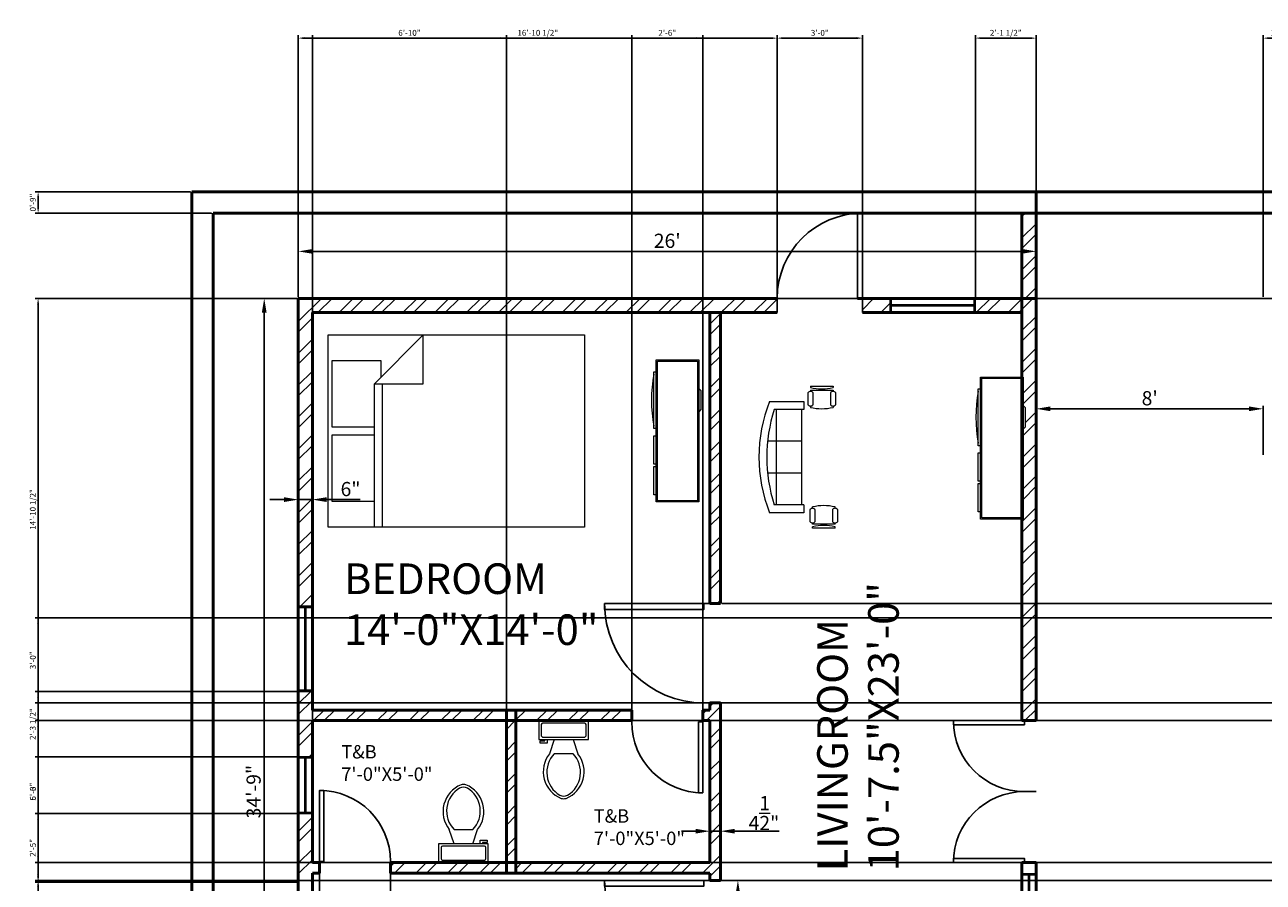
# Model space of a CAD drawing. Units: inches. Extents: x -12550 to 6516, y 1273 to 18700.
# Tile 5 of 19: x 1902 to 2426, y 2226 to 2589. Entities that reach past the tile are written whole.
import ezdxf

# ---------------------------------------------------------------- set-up
doc = ezdxf.new("R2010")
doc.units = ezdxf.units.IN
for name, color, linetype, lineweight in [('A-ANNO-DIMS', 2, 'Continuous', 18), ('A-AREA-IDEN', 1, 'Continuous', 18), ('A-DOOR', 5, 'Continuous', 25), ('A-FURN', 8, 'Continuous', 18), ('A-GLAZ', 3, 'Continuous', 25), ('A-WALL', 7, 'Continuous', 50), ('A-WALL-PATT', 8, 'Continuous', 13)]:
    doc.layers.add(name, color=color, linetype=linetype, lineweight=lineweight)
doc.styles.get("Standard").update_dxf_attribs({"font": 'arial.ttf'})
doc.dimstyles.new('ISO-25', dxfattribs={"dimtxt": 2.5, "dimasz": 2.5, "dimexe": 1.25, "dimexo": 0.625, "dimtad": 1, "dimlunit": 4, "dimtxsty": 'Standard', "dimcen": 2.5, "dimadec": 0, "dimazin": 0, "dimtfac": 1, "dimtmove": 0, "dimatfit": 3, "dimfxl": 1, "dimarcsym": 0})
pattern_1 = [(45, (-2e-13, 567), (-6.735192, 6.735192), []), (45, (4.49, 567), (-6.735192, 6.735192), [])]

# ---------------------------------------------------------------- blocks, each defined once
blk = doc.blocks.new('*U2')
for p, q in [((0, 0), (0, -5)), ((30, 0), (30, -5))]:
    blk.add_line(p, q)
blk.add_lwpolyline([(0, 0), (0, 30), (1.75, 30), (1.75, 0)], close=True)
blk.add_arc((0, 0), 30, 0, 90)
blk = doc.blocks.new('Bed - Queen')
for p, q in [((0, -80.00003), (0, 0)), ((0, 0), (59.99999, 0)), ((59.99999, 0), (59.99999, -80.00003)), ((7.99999, -1.2), (28.79998, -1.2)), ((7.99999, -14.4), (7.99999, -1.2)), ((28.79998, -1.2), (28.79998, -14.4)), ((31.19999, -1.2), (51.99999, -1.2)), ((31.19999, -14.4), (31.19999, -1.2)), ((51.99999, -1.2), (51.99999, -16.4)), ((0, -14.4), (44.8, -14.4)), ((59.99999, -29.6), (44.8, -14.4)), ((44.8, -14.4), (44.8, -29.6)), ((44.8, -16.8), (0, -16.8)), ((51.99999, -16.4), (46.79936, -16.4)), ((44.8, -29.6), (59.99999, -29.6)), ((59.99999, -80.00003), (0, -80.00003))]:
    blk.add_line(p, q)
blk = doc.blocks.new('Toilet - top')
for p, q in [((9.5, -6), (9.5, -2)), ((-10, -8.5), (-8, -8.5)), ((-10, -9.5), (-10, -8.5)), ((-7, -9.5), (-10, -9.5)), ((-8, -8.5), (-8, -8)), ((-7, -8), (-7, -9.5)), ((-4, -8), (-6, -14)), ((4, -8), (6, -14)), ((4, -14), (-4, -14))]:
    blk.add_line(p, q)
blk.add_lwpolyline([(10.5, -8), (10.5, 0), (-10.5, 0), (-10.5, -8)], close=True)
for points in [[(-9.5, -2), (-9.5, -6)], [(8.5, -1), (-8.5, -1)], [(-8.5, -7), (8.5, -7)]]:
    blk.add_lwpolyline(points)
for centre, radius, start, end in [((-8.62, -1.88), 0.884, 81.8699, 188.1301), ((8.62, -1.88), 0.884, 351.8699, 98.1301), ((-8.62, -6.12), 0.884, 171.8699, 278.1301), ((8.62, -6.12), 0.884, 261.8699, 8.1301), ((3.52, -21.58), 12.17, 141.4691, 247.9714), ((4.2, -21.82), 11.33, 136.3677, 238.9468), ((-3.52, -21.58), 12.17, 292.0284, 38.5307), ((-4.2, -21.82), 11.33, 301.053, 43.6321), ((0, -27.88), 4, 245.7318, 294.2682), ((0, -29), 4, 254.8605, 285.1395)]:
    blk.add_arc(centre, radius, start, end)
blk = doc.blocks.new('Entertainment Center')
for p, q in [((-4, 0), (-5, -1)), ((4, 0), (-4, 0)), ((5, -1), (4, 0)), ((-17, -19), (-17, -1)), ((-17, -1), (43, -1)), ((-16.5, -18.5), (-16.5, -1.5)), ((-16.5, -1.5), (42.5, -1.5)), ((42.5, -1.5), (42.5, -18.5)), ((43, -1), (43, -19)), ((43, -19), (-17, -19)), ((42.5, -18.5), (-16.5, -18.5)), ((-12, -20), (-12, -19)), ((12, -20), (-12, -20)), ((12, -19), (12, -20)), ((15, -20), (15, -19)), ((27, -20), (15, -20)), ((27, -19), (27, -20)), ((28, -20), (28, -19)), ((40, -20), (28, -20)), ((40, -19), (40, -20))]:
    blk.add_line(p, q)
blk.add_arc((0, 40), 61, 259.6111, 280.3889)
blk = doc.blocks.new('Sofa - Roundback 7 ft.')
for p, q in [((-12.00002, -32.4421), (-12.00003, -6.5971)), ((11.99997, -32.4421), (11.99998, -6.5971)), ((-36.000027, -34), (-36.000027, -11.4696)), ((-35.999844, -13.3819), (35.9998, -13.3819)), ((35.99998, -34), (35.99998, -11.4696)), ((-36.000027, -32.4421), (35.99998, -32.4421))]:
    blk.add_line(p, q)
for points in [[(-36.000027, -34), (-42.000027, -34), (-42.000027, -8)], [(41.99998, -8), (41.99998, -34), (35.99998, -34)]]:
    blk.add_lwpolyline(points)
for centre, radius, start, end in [((0, -114.25), 114.25, 68.43141, 111.5686), ((-0.00001, -127.1968), 121.1968, 72.72033, 107.2797)]:
    blk.add_arc(centre, radius, start, end)
blk = doc.blocks.new('Chair - Desk')
for p, q in [((-8.5, 0), (-8.5, -1)), ((-8.5, 0), (8.5, 0)), ((8.5, 0), (8.5, -1)), ((-10.5, -5), (-10.5, -14)), ((-8.5, -3), (-8.5, -4)), ((-8.5, -3), (8.5, -3)), ((-6.5, -14), (-6.5, -5)), ((-2, -3), (-2, -1.9355)), ((2, -1.9576), (2, -3)), ((6.5, -5), (6.5, -14)), ((8.5, -3), (8.5, -4)), ((10.5, -14), (10.5, -5)), ((-8.5, -15), (-8.5, -16)), ((8.5, -15), (8.5, -16))]:
    blk.add_line(p, q)
for centre, radius, start, end in [((-8.5, -6.5), 2.5, 36.8699, 143.1301), ((0, 34.625), 36.625, 256.5803, 283.4197), ((8.5, -6.5), 2.5, 36.8699, 143.1301), ((-8.5, -12.5), 2.5, 216.8699, 323.1301), ((0, 19.625), 36.625, 256.5803, 283.4197), ((8.5, -12.5), 2.5, 216.8699, 323.1301)]:
    blk.add_arc(centre, radius, start, end)
blk = doc.blocks.new('*D8')
at = {"layer": 'A-ANNO-DIMS', "color": 0, "lineweight": -2, "transparency": 16777216}
for p, q in [((2011.69, 2388.18), (2005.69, 2388.18)), ((2017.69, 2388.03), (2017.69, 2389.43)), ((2017.69, 2388.18), (2023.69, 2388.18)), ((2023.69, 2388.03), (2023.69, 2389.43)), ((2029.69, 2388.18), (2043.87, 2388.18))]:
    blk.add_line(p, q, dxfattribs=at)
at = {"layer": 'A-ANNO-DIMS', "color": 0, "transparency": 16777216}
for points in [[(2011.69, 2389.18), (2011.69, 2387.18), (2017.69, 2388.18)], [(2029.69, 2389.18), (2029.69, 2387.18), (2023.69, 2388.18)]]:
    blk.add_solid(points, dxfattribs=at)
at = {"layer": 'Defpoints', "color": 0, "transparency": 16777216}
for p in [(2023.69, 2388.18), (2017.69, 2387.4), (2023.69, 2387.4)]:
    blk.add_point(p, dxfattribs=at)
at = {"layer": 'A-ANNO-DIMS', "color": 0, "transparency": 16777216, "insert": (2039.78, 2391.87), "char_height": 6, "attachment_point": 5}
blk.add_mtext('6"', dxfattribs=at)
blk = doc.blocks.new('*D9')
at = {"layer": 'A-ANNO-DIMS', "color": 0, "lineweight": -2, "transparency": 16777216}
for p, q in [((2191.69, 2251.78), (2191.69, 2246.78)), ((2196.19, 2251.78), (2196.19, 2246.78)), ((2185.69, 2248.03), (2179.69, 2248.03)), ((2191.69, 2248.03), (2196.19, 2248.03)), ((2202.19, 2248.03), (2220.95, 2248.03))]:
    blk.add_line(p, q, dxfattribs=at)
at = {"layer": 'A-ANNO-DIMS', "color": 0, "transparency": 16777216}
for points in [[(2185.69, 2249.03), (2185.69, 2247.03), (2191.69, 2248.03)], [(2202.19, 2249.03), (2202.19, 2247.03), (2196.19, 2248.03)]]:
    blk.add_solid(points, dxfattribs=at)
at = {"layer": 'Defpoints', "color": 0, "transparency": 16777216}
for p in [(2191.69, 2252.41), (2196.19, 2252.41), (2196.19, 2248.03)]:
    blk.add_point(p, dxfattribs=at)
at = {"layer": 'A-ANNO-DIMS', "color": 0, "transparency": 16777216, "insert": (2214.57, 2255.68), "char_height": 6, "attachment_point": 5}
blk.add_mtext('4{\\H1x;\\S1/2;}"', dxfattribs=at)
blk = doc.blocks.new('*D10')
at = {"layer": 'A-ANNO-DIMS', "color": 0, "lineweight": -2, "transparency": 16777216}
for p, q in [((2196.81, 2227.25), (2204.82, 2227.25)), ((2203.57, 2221.25), (2203.57, 2191.25)), ((2196.81, 2185.25), (2204.82, 2185.25))]:
    blk.add_line(p, q, dxfattribs=at)
at = {"layer": 'A-ANNO-DIMS', "color": 0, "transparency": 16777216}
for points in [[(2202.57, 2221.25), (2204.57, 2221.25), (2203.57, 2227.25)], [(2202.57, 2191.25), (2204.57, 2191.25), (2203.57, 2185.25)]]:
    blk.add_solid(points, dxfattribs=at)
at = {"layer": 'Defpoints', "color": 0, "transparency": 16777216}
for p in [(2196.19, 2227.25), (2196.19, 2185.25), (2203.57, 2185.25)]:
    blk.add_point(p, dxfattribs=at)
at = {"layer": 'A-ANNO-DIMS', "color": 0, "transparency": 16777216, "insert": (2199.88, 2206.25), "char_height": 6, "attachment_point": 5, "rotation": 90}
blk.add_mtext('3\'-6"', dxfattribs=at)
blk = doc.blocks.new('*D15')
at = {"layer": 'A-ANNO-DIMS', "color": 0, "lineweight": -2, "transparency": 16777216}
for p, q in [((2017.06, 2473.25), (2002.03, 2473.25)), ((2003.28, 2467.25), (2003.28, 2062.25)), ((2017.06, 2056.25), (2002.03, 2056.25))]:
    blk.add_line(p, q, dxfattribs=at)
at = {"layer": 'A-ANNO-DIMS', "color": 0, "transparency": 16777216}
for points in [[(2002.28, 2467.25), (2004.28, 2467.25), (2003.28, 2473.25)], [(2002.28, 2062.25), (2004.28, 2062.25), (2003.28, 2056.25)]]:
    blk.add_solid(points, dxfattribs=at)
at = {"layer": 'Defpoints', "color": 0, "transparency": 16777216}
for p in [(2017.69, 2473.25), (2003.28, 2056.25), (2017.69, 2056.25)]:
    blk.add_point(p, dxfattribs=at)
at = {"layer": 'A-ANNO-DIMS', "color": 0, "transparency": 16777216, "insert": (1999.59, 2264.75), "char_height": 6, "attachment_point": 5, "rotation": 90}
blk.add_mtext('34\'-9"', dxfattribs=at)
blk = doc.blocks.new('*D18')
at = {"layer": 'A-ANNO-DIMS', "color": 0, "lineweight": -2, "transparency": 16777216}
for p, q in [((2017.69, 2473.87), (2017.69, 2494.36)), ((2023.69, 2493.11), (2323.69, 2493.11)), ((2329.69, 2473.87), (2329.69, 2494.36))]:
    blk.add_line(p, q, dxfattribs=at)
at = {"layer": 'A-ANNO-DIMS', "color": 0, "transparency": 16777216}
for points in [[(2023.69, 2494.11), (2023.69, 2492.11), (2017.69, 2493.11)], [(2323.69, 2494.11), (2323.69, 2492.11), (2329.69, 2493.11)]]:
    blk.add_solid(points, dxfattribs=at)
at = {"layer": 'Defpoints', "color": 0, "transparency": 16777216}
for p in [(2329.69, 2493.11), (2017.69, 2473.25), (2329.69, 2473.25)]:
    blk.add_point(p, dxfattribs=at)
at = {"layer": 'A-ANNO-DIMS', "color": 0, "transparency": 16777216, "insert": (2173.69, 2496.8), "char_height": 6, "attachment_point": 5}
blk.add_mtext("26'", dxfattribs=at)
blk = doc.blocks.new('*D19')
at = {"layer": 'A-ANNO-DIMS', "color": 0, "lineweight": -2, "transparency": 16777216}
for p, q in [((2329.69, 2407.12), (2329.69, 2427.81)), ((2335.69, 2426.56), (2419.69, 2426.56)), ((2425.69, 2407.12), (2425.69, 2427.81))]:
    blk.add_line(p, q, dxfattribs=at)
at = {"layer": 'A-ANNO-DIMS', "color": 0, "transparency": 16777216}
for points in [[(2335.69, 2427.56), (2335.69, 2425.56), (2329.69, 2426.56)], [(2419.69, 2427.56), (2419.69, 2425.56), (2425.69, 2426.56)]]:
    blk.add_solid(points, dxfattribs=at)
at = {"layer": 'Defpoints', "color": 0, "transparency": 16777216}
for p in [(2425.69, 2426.56), (2329.69, 2406.5), (2425.69, 2406.5)]:
    blk.add_point(p, dxfattribs=at)
at = {"layer": 'A-ANNO-DIMS', "color": 0, "transparency": 16777216, "insert": (2377.69, 2430.25), "char_height": 6, "attachment_point": 5}
blk.add_mtext("8'", dxfattribs=at)
blk = doc.blocks.new('WIN-3FT')
for p, q in [((0, 0), (0, 6)), ((0, 6), (36.02, 6)), ((0.5, 0), (0.5, 6)), ((35.52, 6), (35.52, 0)), ((36.02, 6), (36.02, 0)), ((36.02, 0), (0, 0)), ((35.52, 3.2), (0.5, 3.2)), ((35.52, 2.8), (0.5, 2.8))]:
    blk.add_line(p, q)
blk = doc.blocks.new('WIN-2FT')
for p, q in [((0, 0), (0, 24.02)), ((0, 24.02), (6, 24.02)), ((0, 23.52), (6, 23.52)), ((2.8, 0.5), (2.8, 23.52)), ((3.2, 0.5), (3.2, 23.52)), ((6, 24.02), (6, 0)), ((6, 0.5), (0, 0.5)), ((6, 0), (0, 0))]:
    blk.add_line(p, q)
blk = doc.blocks.new('*D102')
at = {"layer": 'A-ANNO-DIMS', "color": 0, "lineweight": -2, "transparency": 16777216}
for p, q in [((1972.06, 2518.25), (1906.44, 2518.25)), ((1907.69, 2515.75), (1907.69, 2511.75)), ((1981.06, 2509.25), (1906.44, 2509.25))]:
    blk.add_line(p, q, dxfattribs=at)
at = {"layer": 'A-ANNO-DIMS', "color": 0, "transparency": 16777216}
for points in [[(1907.27, 2515.75), (1908.11, 2515.75), (1907.69, 2518.25)], [(1907.27, 2511.75), (1908.11, 2511.75), (1907.69, 2509.25)]]:
    blk.add_solid(points, dxfattribs=at)
at = {"layer": 'Defpoints', "color": 0, "transparency": 16777216}
for p in [(1972.69, 2518.25), (1907.69, 2509.25), (1981.69, 2509.25)]:
    blk.add_point(p, dxfattribs=at)
at = {"layer": 'A-ANNO-DIMS', "color": 0, "transparency": 16777216, "insert": (1905.79, 2513.75), "char_height": 2.5, "attachment_point": 5, "rotation": 90}
blk.add_mtext('0\'-9"', dxfattribs=at)
blk = doc.blocks.new('*D130')
at = {"layer": 'A-ANNO-DIMS', "color": 0, "lineweight": -2, "transparency": 16777216}
for p, q in [((2017.69, 2473.87), (2017.69, 2584.5)), ((2020.19, 2583.25), (2217.69, 2583.25)), ((2220.19, 2473.87), (2220.19, 2584.5))]:
    blk.add_line(p, q, dxfattribs=at)
at = {"layer": 'A-ANNO-DIMS', "color": 0, "transparency": 16777216}
for points in [[(2020.19, 2583.66), (2020.19, 2582.83), (2017.69, 2583.25)], [(2217.69, 2583.66), (2217.69, 2582.83), (2220.19, 2583.25)]]:
    blk.add_solid(points, dxfattribs=at)
at = {"layer": 'Defpoints', "color": 0, "transparency": 16777216}
for p in [(2220.19, 2583.25), (2017.69, 2473.25), (2220.19, 2473.25)]:
    blk.add_point(p, dxfattribs=at)
at = {"layer": 'A-ANNO-DIMS', "color": 0, "transparency": 16777216, "insert": (2118.94, 2585.16), "char_height": 2.5, "attachment_point": 5}
blk.add_mtext('16\'-10 1/2"', dxfattribs=at)
blk = doc.blocks.new('*D131')
at = {"layer": 'A-ANNO-DIMS', "color": 0, "lineweight": -2, "transparency": 16777216}
for p, q in [((2220.19, 2473.87), (2220.19, 2584.5)), ((2222.69, 2583.25), (2253.69, 2583.25)), ((2256.19, 2473.87), (2256.19, 2584.5))]:
    blk.add_line(p, q, dxfattribs=at)
at = {"layer": 'A-ANNO-DIMS', "color": 0, "transparency": 16777216}
for points in [[(2222.69, 2583.66), (2222.69, 2582.83), (2220.19, 2583.25)], [(2253.69, 2583.66), (2253.69, 2582.83), (2256.19, 2583.25)]]:
    blk.add_solid(points, dxfattribs=at)
at = {"layer": 'Defpoints', "color": 0, "transparency": 16777216}
for p in [(2256.19, 2583.25), (2220.19, 2473.25), (2256.19, 2473.25)]:
    blk.add_point(p, dxfattribs=at)
at = {"layer": 'A-ANNO-DIMS', "color": 0, "transparency": 16777216, "insert": (2238.19, 2585.15), "char_height": 2.5, "attachment_point": 5}
blk.add_mtext('3\'-0"', dxfattribs=at)
blk = doc.blocks.new('*D132')
at = {"layer": 'A-ANNO-DIMS', "color": 0, "lineweight": -2, "transparency": 16777216}
for p, q in [((2303.96, 2473.87), (2303.96, 2584.5)), ((2306.46, 2583.25), (2327.19, 2583.25)), ((2329.69, 2473.87), (2329.69, 2584.5))]:
    blk.add_line(p, q, dxfattribs=at)
at = {"layer": 'A-ANNO-DIMS', "color": 0, "transparency": 16777216}
for points in [[(2306.46, 2583.66), (2306.46, 2582.83), (2303.96, 2583.25)], [(2327.19, 2583.66), (2327.19, 2582.83), (2329.69, 2583.25)]]:
    blk.add_solid(points, dxfattribs=at)
at = {"layer": 'Defpoints', "color": 0, "transparency": 16777216}
for p in [(2329.69, 2583.25), (2303.96, 2473.25), (2329.69, 2473.25)]:
    blk.add_point(p, dxfattribs=at)
at = {"layer": 'A-ANNO-DIMS', "color": 0, "transparency": 16777216, "insert": (2316.82, 2585.16), "char_height": 2.5, "attachment_point": 5}
blk.add_mtext('2\'-1 1/2"', dxfattribs=at)
blk = doc.blocks.new('*D134')
at = {"layer": 'A-ANNO-DIMS', "color": 0, "lineweight": -2, "transparency": 16777216}
for p, q in [((2017.06, 2255.45), (1906.44, 2255.45)), ((1907.69, 2228.95), (1907.69, 2252.95)), ((2017.06, 2226.45), (1906.44, 2226.45))]:
    blk.add_line(p, q, dxfattribs=at)
at = {"layer": 'A-ANNO-DIMS', "color": 0, "transparency": 16777216}
for points in [[(1907.27, 2252.95), (1908.11, 2252.95), (1907.69, 2255.45)], [(1907.27, 2228.95), (1908.11, 2228.95), (1907.69, 2226.45)]]:
    blk.add_solid(points, dxfattribs=at)
at = {"layer": 'Defpoints', "color": 0, "transparency": 16777216}
for p in [(1907.69, 2255.45), (2017.69, 2255.45), (2017.69, 2226.45)]:
    blk.add_point(p, dxfattribs=at)
at = {"layer": 'A-ANNO-DIMS', "color": 0, "transparency": 16777216, "insert": (1905.79, 2240.95), "char_height": 2.5, "attachment_point": 5, "rotation": 90}
blk.add_mtext('2\'-5"', dxfattribs=at)
blk = doc.blocks.new('*D135')
at = {"layer": 'A-ANNO-DIMS', "color": 0, "lineweight": -2, "transparency": 16777216}
for p, q in [((2017.06, 2307.12), (1906.44, 2307.12)), ((1907.69, 2281.97), (1907.69, 2304.62)), ((2017.06, 2279.47), (1906.44, 2279.47))]:
    blk.add_line(p, q, dxfattribs=at)
at = {"layer": 'A-ANNO-DIMS', "color": 0, "transparency": 16777216}
for points in [[(1907.27, 2304.62), (1908.11, 2304.62), (1907.69, 2307.12)], [(1907.27, 2281.97), (1908.11, 2281.97), (1907.69, 2279.47)]]:
    blk.add_solid(points, dxfattribs=at)
at = {"layer": 'Defpoints', "color": 0, "transparency": 16777216}
for p in [(1907.69, 2307.12), (2017.69, 2307.12), (2017.69, 2279.47)]:
    blk.add_point(p, dxfattribs=at)
at = {"layer": 'A-ANNO-DIMS', "color": 0, "transparency": 16777216, "insert": (1905.77, 2293.29), "char_height": 2.5, "attachment_point": 5, "rotation": 90}
blk.add_mtext('2\'-3 1/2"', dxfattribs=at)
blk = doc.blocks.new('*D139')
at = {"layer": 'A-ANNO-DIMS', "color": 0, "lineweight": -2, "transparency": 16777216}
for p, q in [((2196.81, 2302.25), (2848.94, 2302.25)), ((2847.69, 2229.75), (2847.69, 2299.75)), ((2196.81, 2227.25), (2848.94, 2227.25))]:
    blk.add_line(p, q, dxfattribs=at)
at = {"layer": 'A-ANNO-DIMS', "color": 0, "transparency": 16777216}
for points in [[(2847.27, 2299.75), (2848.11, 2299.75), (2847.69, 2302.25)], [(2847.27, 2229.75), (2848.11, 2229.75), (2847.69, 2227.25)]]:
    blk.add_solid(points, dxfattribs=at)
at = {"layer": 'Defpoints', "color": 0, "transparency": 16777216}
for p in [(2196.19, 2302.25), (2847.69, 2302.25), (2196.19, 2227.25)]:
    blk.add_point(p, dxfattribs=at)
at = {"layer": 'A-ANNO-DIMS', "color": 0, "transparency": 16777216, "insert": (2845.79, 2264.75), "char_height": 2.5, "attachment_point": 5, "rotation": 90}
blk.add_mtext('6\'-3"', dxfattribs=at)
blk = doc.blocks.new('*D140')
at = {"layer": 'A-ANNO-DIMS', "color": 0, "lineweight": -2, "transparency": 16777216}
for p, q in [((2196.81, 2344.25), (2848.94, 2344.25)), ((2847.69, 2304.75), (2847.69, 2341.75)), ((2196.81, 2302.25), (2848.94, 2302.25))]:
    blk.add_line(p, q, dxfattribs=at)
at = {"layer": 'A-ANNO-DIMS', "color": 0, "transparency": 16777216}
for points in [[(2847.27, 2341.75), (2848.11, 2341.75), (2847.69, 2344.25)], [(2847.27, 2304.75), (2848.11, 2304.75), (2847.69, 2302.25)]]:
    blk.add_solid(points, dxfattribs=at)
at = {"layer": 'Defpoints', "color": 0, "transparency": 16777216}
for p in [(2196.19, 2344.25), (2847.69, 2344.25), (2196.19, 2302.25)]:
    blk.add_point(p, dxfattribs=at)
at = {"layer": 'A-ANNO-DIMS', "color": 0, "transparency": 16777216, "insert": (2845.79, 2323.25), "char_height": 2.5, "attachment_point": 5, "rotation": 90}
blk.add_mtext('3\'-6"', dxfattribs=at)
blk = doc.blocks.new('*D141')
at = {"layer": 'A-ANNO-DIMS', "color": 0, "lineweight": -2, "transparency": 16777216}
for p, q in [((2158.69, 2295.37), (2158.69, 2584.5)), ((2161.19, 2583.25), (2186.19, 2583.25)), ((2188.69, 2295.37), (2188.69, 2584.5))]:
    blk.add_line(p, q, dxfattribs=at)
at = {"layer": 'A-ANNO-DIMS', "color": 0, "transparency": 16777216}
for points in [[(2161.19, 2583.66), (2161.19, 2582.83), (2158.69, 2583.25)], [(2186.19, 2583.66), (2186.19, 2582.83), (2188.69, 2583.25)]]:
    blk.add_solid(points, dxfattribs=at)
at = {"layer": 'Defpoints', "color": 0, "transparency": 16777216}
for p in [(2188.69, 2583.25), (2158.69, 2294.75), (2188.69, 2294.75)]:
    blk.add_point(p, dxfattribs=at)
at = {"layer": 'A-ANNO-DIMS', "color": 0, "transparency": 16777216, "insert": (2173.69, 2585.15), "char_height": 2.5, "attachment_point": 5}
blk.add_mtext('2\'-6"', dxfattribs=at)
blk = doc.blocks.new('*D142')
at = {"layer": 'A-ANNO-DIMS', "color": 0, "lineweight": -2, "transparency": 16777216}
for p, q in [((2026.69, 2234.12), (2026.69, 1378)), ((2056.69, 2234.12), (2056.69, 1378)), ((2029.19, 1379.25), (2054.19, 1379.25))]:
    blk.add_line(p, q, dxfattribs=at)
at = {"layer": 'A-ANNO-DIMS', "color": 0, "transparency": 16777216}
for points in [[(2029.19, 1379.66), (2029.19, 1378.83), (2026.69, 1379.25)], [(2054.19, 1379.66), (2054.19, 1378.83), (2056.69, 1379.25)]]:
    blk.add_solid(points, dxfattribs=at)
at = {"layer": 'Defpoints', "color": 0, "transparency": 16777216}
for p in [(2026.69, 2234.75), (2056.69, 2234.75), (2056.69, 1379.25)]:
    blk.add_point(p, dxfattribs=at)
at = {"layer": 'A-ANNO-DIMS', "color": 0, "transparency": 16777216, "insert": (2041.69, 1381.15), "char_height": 2.5, "attachment_point": 5}
blk.add_mtext('2\'-6"', dxfattribs=at)
blk = doc.blocks.new('*D143')
at = {"layer": 'A-ANNO-DIMS', "color": 0, "lineweight": -2, "transparency": 16777216}
for p, q in [((2023.69, 2295.37), (2023.69, 2584.5)), ((2026.19, 2583.25), (2103.19, 2583.25)), ((2105.69, 2299.87), (2105.69, 2584.5))]:
    blk.add_line(p, q, dxfattribs=at)
at = {"layer": 'A-ANNO-DIMS', "color": 0, "transparency": 16777216}
for points in [[(2026.19, 2583.66), (2026.19, 2582.83), (2023.69, 2583.25)], [(2103.19, 2583.66), (2103.19, 2582.83), (2105.69, 2583.25)]]:
    blk.add_solid(points, dxfattribs=at)
at = {"layer": 'Defpoints', "color": 0, "transparency": 16777216}
for p in [(2105.69, 2583.25), (2105.69, 2299.25), (2023.69, 2294.75)]:
    blk.add_point(p, dxfattribs=at)
at = {"layer": 'A-ANNO-DIMS', "color": 0, "transparency": 16777216, "insert": (2064.69, 2585.15), "char_height": 2.5, "attachment_point": 5}
blk.add_mtext('6\'-10"', dxfattribs=at)
blk = doc.blocks.new('*D144')
at = {"layer": 'A-ANNO-DIMS', "color": 0, "lineweight": -2, "transparency": 16777216}
for p, q in [((2330.31, 2294.75), (2848.94, 2294.75)), ((2847.69, 2237.25), (2847.69, 2292.25)), ((2330.31, 2234.75), (2848.94, 2234.75))]:
    blk.add_line(p, q, dxfattribs=at)
at = {"layer": 'A-ANNO-DIMS', "color": 0, "transparency": 16777216}
for points in [[(2847.27, 2292.25), (2848.11, 2292.25), (2847.69, 2294.75)], [(2847.27, 2237.25), (2848.11, 2237.25), (2847.69, 2234.75)]]:
    blk.add_solid(points, dxfattribs=at)
at = {"layer": 'Defpoints', "color": 0, "transparency": 16777216}
for p in [(2329.69, 2294.75), (2847.69, 2294.75), (2329.69, 2234.75)]:
    blk.add_point(p, dxfattribs=at)
at = {"layer": 'A-ANNO-DIMS', "color": 0, "transparency": 16777216, "insert": (2845.79, 2264.75), "char_height": 2.5, "attachment_point": 5, "rotation": 90}
blk.add_mtext('5\'-0"', dxfattribs=at)
blk = doc.blocks.new('*D146')
at = {"layer": 'A-ANNO-DIMS', "color": 0, "lineweight": -2, "transparency": 16777216}
for p, q in [((2330.31, 2473.25), (2848.94, 2473.25)), ((2847.69, 2297.25), (2847.69, 2470.75)), ((2330.31, 2294.75), (2848.94, 2294.75))]:
    blk.add_line(p, q, dxfattribs=at)
at = {"layer": 'A-ANNO-DIMS', "color": 0, "transparency": 16777216}
for points in [[(2847.27, 2470.75), (2848.11, 2470.75), (2847.69, 2473.25)], [(2847.27, 2297.25), (2848.11, 2297.25), (2847.69, 2294.75)]]:
    blk.add_solid(points, dxfattribs=at)
at = {"layer": 'Defpoints', "color": 0, "transparency": 16777216}
for p in [(2329.69, 2473.25), (2847.69, 2473.25), (2329.69, 2294.75)]:
    blk.add_point(p, dxfattribs=at)
at = {"layer": 'A-ANNO-DIMS', "color": 0, "transparency": 16777216, "insert": (2845.77, 2384), "char_height": 2.5, "attachment_point": 5, "rotation": 90}
blk.add_mtext('14\'-10 1/2"', dxfattribs=at)
blk = doc.blocks.new('*D149')
at = {"layer": 'A-ANNO-DIMS', "color": 0, "lineweight": -2, "transparency": 16777216}
for p, q in [((2425.69, 2473.87), (2425.69, 2584.5)), ((2428.19, 2583.25), (2436.95, 2583.25)), ((2439.45, 2473.87), (2439.45, 2584.5))]:
    blk.add_line(p, q, dxfattribs=at)
at = {"layer": 'A-ANNO-DIMS', "color": 0, "transparency": 16777216}
for points in [[(2428.19, 2583.66), (2428.19, 2582.83), (2425.69, 2583.25)], [(2436.95, 2583.66), (2436.95, 2582.83), (2439.45, 2583.25)]]:
    blk.add_solid(points, dxfattribs=at)
at = {"layer": 'Defpoints', "color": 0, "transparency": 16777216}
for p in [(2439.45, 2583.25), (2425.69, 2473.25), (2439.45, 2473.25)]:
    blk.add_point(p, dxfattribs=at)
at = {"layer": 'A-ANNO-DIMS', "color": 0, "transparency": 16777216, "insert": (2432.57, 2585.13), "char_height": 2.5, "attachment_point": 5}
blk.add_mtext('1\'-2"', dxfattribs=at)
blk = doc.blocks.new('*D158')
at = {"layer": 'A-ANNO-DIMS', "color": 0, "lineweight": -2, "transparency": 16777216}
for p, q in [((2558.56, 2227.25), (1906.44, 2227.25)), ((1907.69, 2193.75), (1907.69, 2224.75)), ((2558.56, 2191.25), (1906.44, 2191.25))]:
    blk.add_line(p, q, dxfattribs=at)
at = {"layer": 'A-ANNO-DIMS', "color": 0, "transparency": 16777216}
for points in [[(1907.27, 2224.75), (1908.11, 2224.75), (1907.69, 2227.25)], [(1907.27, 2193.75), (1908.11, 2193.75), (1907.69, 2191.25)]]:
    blk.add_solid(points, dxfattribs=at)
at = {"layer": 'Defpoints', "color": 0, "transparency": 16777216}
for p in [(1907.69, 2227.25), (2559.19, 2227.25), (2559.19, 2191.25)]:
    blk.add_point(p, dxfattribs=at)
at = {"layer": 'A-ANNO-DIMS', "color": 0, "transparency": 16777216, "insert": (1905.79, 2209.25), "char_height": 2.5, "attachment_point": 5, "rotation": 90}
blk.add_mtext('3\'-0"', dxfattribs=at)
blk = doc.blocks.new('*D159')
at = {"layer": 'A-ANNO-DIMS', "color": 0, "lineweight": -2, "transparency": 16777216}
for p, q in [((2558.56, 2302.25), (1906.44, 2302.25)), ((1907.69, 2229.75), (1907.69, 2299.75)), ((2558.56, 2227.25), (1906.44, 2227.25))]:
    blk.add_line(p, q, dxfattribs=at)
at = {"layer": 'A-ANNO-DIMS', "color": 0, "transparency": 16777216}
for points in [[(1907.27, 2299.75), (1908.11, 2299.75), (1907.69, 2302.25)], [(1907.27, 2229.75), (1908.11, 2229.75), (1907.69, 2227.25)]]:
    blk.add_solid(points, dxfattribs=at)
at = {"layer": 'Defpoints', "color": 0, "transparency": 16777216}
for p in [(1907.69, 2302.25), (2559.19, 2302.25), (2559.19, 2227.25)]:
    blk.add_point(p, dxfattribs=at)
at = {"layer": 'A-ANNO-DIMS', "color": 0, "transparency": 16777216, "insert": (1905.79, 2264.75), "char_height": 2.5, "attachment_point": 5, "rotation": 90}
blk.add_mtext('6\'-3"', dxfattribs=at)
blk = doc.blocks.new('*D160')
at = {"layer": 'A-ANNO-DIMS', "color": 0, "lineweight": -2, "transparency": 16777216}
for p, q in [((2558.56, 2338.25), (1906.44, 2338.25)), ((1907.69, 2304.75), (1907.69, 2335.75)), ((2558.56, 2302.25), (1906.44, 2302.25))]:
    blk.add_line(p, q, dxfattribs=at)
at = {"layer": 'A-ANNO-DIMS', "color": 0, "transparency": 16777216}
for points in [[(1907.27, 2335.75), (1908.11, 2335.75), (1907.69, 2338.25)], [(1907.27, 2304.75), (1908.11, 2304.75), (1907.69, 2302.25)]]:
    blk.add_solid(points, dxfattribs=at)
at = {"layer": 'Defpoints', "color": 0, "transparency": 16777216}
for p in [(1907.69, 2338.25), (2559.19, 2338.25), (2559.19, 2302.25)]:
    blk.add_point(p, dxfattribs=at)
at = {"layer": 'A-ANNO-DIMS', "color": 0, "transparency": 16777216, "insert": (1905.79, 2320.25), "char_height": 2.5, "attachment_point": 5, "rotation": 90}
blk.add_mtext('3\'-0"', dxfattribs=at)
blk = doc.blocks.new('*D164')
at = {"layer": 'A-ANNO-DIMS', "color": 0, "lineweight": -2, "transparency": 16777216}
for p, q in [((2425.06, 2294.75), (1906.44, 2294.75)), ((1907.69, 2237.25), (1907.69, 2292.25)), ((2425.06, 2234.75), (1906.44, 2234.75))]:
    blk.add_line(p, q, dxfattribs=at)
at = {"layer": 'A-ANNO-DIMS', "color": 0, "transparency": 16777216}
for points in [[(1907.27, 2292.25), (1908.11, 2292.25), (1907.69, 2294.75)], [(1907.27, 2237.25), (1908.11, 2237.25), (1907.69, 2234.75)]]:
    blk.add_solid(points, dxfattribs=at)
at = {"layer": 'Defpoints', "color": 0, "transparency": 16777216}
for p in [(1907.69, 2294.75), (2425.69, 2294.75), (2425.69, 2234.75)]:
    blk.add_point(p, dxfattribs=at)
at = {"layer": 'A-ANNO-DIMS', "color": 0, "transparency": 16777216, "insert": (1905.79, 2264.75), "char_height": 2.5, "attachment_point": 5, "rotation": 90}
blk.add_mtext('5\'-0"', dxfattribs=at)
blk = doc.blocks.new('*D166')
at = {"layer": 'A-ANNO-DIMS', "color": 0, "lineweight": -2, "transparency": 16777216}
for p, q in [((2425.06, 2473.25), (1906.44, 2473.25)), ((1907.69, 2297.25), (1907.69, 2470.75)), ((2425.06, 2294.75), (1906.44, 2294.75))]:
    blk.add_line(p, q, dxfattribs=at)
at = {"layer": 'A-ANNO-DIMS', "color": 0, "transparency": 16777216}
for points in [[(1907.27, 2470.75), (1908.11, 2470.75), (1907.69, 2473.25)], [(1907.27, 2297.25), (1908.11, 2297.25), (1907.69, 2294.75)]]:
    blk.add_solid(points, dxfattribs=at)
at = {"layer": 'Defpoints', "color": 0, "transparency": 16777216}
for p in [(1907.69, 2473.25), (2425.69, 2473.25), (2425.69, 2294.75)]:
    blk.add_point(p, dxfattribs=at)
at = {"layer": 'A-ANNO-DIMS', "color": 0, "transparency": 16777216, "insert": (1905.77, 2384), "char_height": 2.5, "attachment_point": 5, "rotation": 90}
blk.add_mtext('14\'-10 1/2"', dxfattribs=at)

msp = doc.modelspace()

# ---------------------------------------------------------------- hatches: boundary and pattern name
at = {"layer": 'A-WALL-PATT'}
h = msp.add_hatch(dxfattribs=at)
h.set_pattern_fill('ANSI32', color=256)
h.paths.add_polyline_path([(2329.689, 2509.247), (2323.689, 2509.247), (2323.689, 2473.247), (2329.689, 2473.247)])
h = msp.add_hatch(dxfattribs=at)
h.set_pattern_fill('ANSI32', color=256)
h.set_pattern_definition(pattern_1)
h.paths.add_polyline_path([(2023.689, 2467.247), (2197.689, 2467.247), (2197.689, 2473.247), (2017.689, 2473.247), (2017.689, 2343.138), (2023.689, 2343.138)])
h = msp.add_hatch(dxfattribs=at)
h.set_pattern_fill('ANSI32', color=256)
h.set_pattern_definition(pattern_1)
h.paths.add_polyline_path([(2256.189, 2473.247), (2256.189, 2467.247), (2267.94, 2467.247), (2267.94, 2473.247)])
h.paths.add_polyline_path([(2220.189, 2467.247), (2220.189, 2473.247), (2197.689, 2473.247), (2197.689, 2467.247)])
h = msp.add_hatch(dxfattribs=at)
h.set_pattern_fill('ANSI32', color=256)
h.set_pattern_definition(pattern_1)
h.paths.add_polyline_path([(2329.689, 2473.247), (2303.958, 2473.247), (2303.958, 2467.247), (2323.689, 2467.247), (2323.689, 2439.972), (2324.189, 2439.972), (2324.189, 2427.972), (2325.189, 2426.972), (2325.189, 2418.972), (2324.189, 2417.972), (2324.189, 2379.972), (2323.689, 2294.747), (2324.689, 2294.747), (2329.689, 2294.747)])
h = msp.add_hatch(dxfattribs=at)
h.set_pattern_fill('ANSI32', color=256)
h.set_pattern_definition(pattern_1)
h.paths.add_polyline_path([(2196.189, 2467.247), (2191.689, 2467.247), (2191.689, 2344.247), (2196.189, 2344.247)], flags=17)
h = msp.add_hatch(dxfattribs=at)
h.set_pattern_fill('ANSI32', color=256)
h.set_pattern_definition(pattern_1)
h.paths.add_polyline_path([(2105.689, 2299.247), (2023.689, 2299.247), (2023.689, 2307.121), (2017.689, 2307.121), (2017.689, 2279.466), (2023.689, 2279.466), (2023.689, 2294.747), (2105.689, 2294.747)])
h = msp.add_hatch(dxfattribs=at)
h.set_pattern_fill('ANSI32', color=256)
h.set_pattern_definition(pattern_1)
h.paths.add_polyline_path([(2196.189, 2302.247), (2191.689, 2302.247), (2191.689, 2299.247), (2188.689, 2299.247), (2188.689, 2294.747), (2191.689, 2294.747), (2191.689, 2234.747), (2109.689, 2234.747), (2109.689, 2230.247), (2191.689, 2230.247), (2191.689, 2227.247), (2196.189, 2227.247)])
h = msp.add_hatch(dxfattribs=at)
h.set_pattern_fill('ANSI32', color=256)
h.set_pattern_definition(pattern_1)
h.paths.add_polyline_path([(2158.689, 2299.247), (2109.689, 2299.247), (2109.689, 2294.747), (2158.689, 2294.747)], flags=17)
h = msp.add_hatch(dxfattribs=at)
h.set_pattern_fill('ANSI32', color=256)
h.set_pattern_definition(pattern_1)
h.paths.add_polyline_path([(2109.689, 2294.747), (2105.689, 2294.747), (2105.689, 2234.747), (2109.689, 2234.747)])
h = msp.add_hatch(dxfattribs=at)
h.set_pattern_fill('ANSI32', color=256)
h.set_pattern_definition(pattern_1)
h.paths.add_polyline_path([(2023.689, 2255.449), (2017.689, 2255.449), (2017.689, 2226.453), (2023.689, 2226.453), (2023.689, 2230.247), (2026.689, 2230.247), (2026.689, 2234.747), (2023.689, 2234.747)])
h = msp.add_hatch(dxfattribs=at)
h.set_pattern_fill('ANSI32', color=256)
h.set_pattern_definition(pattern_1)
h.paths.add_polyline_path([(2105.689, 2234.747), (2056.689, 2234.747), (2056.689, 2230.247), (2105.689, 2230.247)])

# ---------------------------------------------------------------- linework, layer by layer
at = {"layer": 'A-WALL'}
for p, q in [((1972.689, 2518.247), (2782.689, 2518.247)), ((1972.689, 1444.247), (1972.689, 2518.247)), ((2329.689, 2294.747), (2329.689, 2518.247)), ((1981.689, 2509.247), (2773.689, 2509.247)), ((1981.689, 1453.247), (1981.689, 2509.247)), ((2554.089, 2509.247), (2254.089, 2509.247)), ((2323.689, 2294.747), (2323.689, 2509.247)), ((2017.689, 2068.324), (2017.689, 2473.247)), ((2220.189, 2473.247), (2017.689, 2473.247)), ((2329.689, 2473.247), (2254.089, 2473.247)), ((2023.689, 2299.247), (2023.689, 2467.247)), ((2220.189, 2467.247), (2023.689, 2467.247)), ((2191.689, 2344.247), (2191.689, 2467.247)), ((2196.189, 2344.247), (2196.189, 2467.247)), ((2323.689, 2467.247), (2256.189, 2467.247)), ((2196.189, 2344.247), (2191.689, 2344.247)), ((2158.689, 2299.247), (2023.689, 2299.247)), ((2105.689, 2230.247), (2105.689, 2299.247)), ((2109.689, 2230.247), (2109.689, 2299.247)), ((2158.689, 2294.747), (2158.689, 2299.247)), ((2191.689, 2299.247), (2188.689, 2299.247)), ((2191.689, 2299.247), (2188.689, 2299.247)), ((2188.689, 2299.247), (2188.689, 2294.747)), ((2191.689, 2299.247), (2191.689, 2302.247)), ((2191.689, 2299.247), (2191.689, 2302.247)), ((2191.689, 2302.247), (2196.189, 2302.247)), ((2196.189, 2227.247), (2196.189, 2302.247)), ((2158.689, 2294.747), (2023.689, 2294.747)), ((2023.689, 2234.747), (2023.689, 2294.747)), ((2191.689, 2294.747), (2188.689, 2294.747)), ((2191.689, 2234.747), (2191.689, 2294.747)), ((2329.689, 2294.747), (2323.689, 2294.747)), ((2026.689, 2234.747), (2023.689, 2234.747)), ((2026.689, 2230.247), (2026.689, 2234.747)), ((2191.689, 2234.747), (2056.689, 2234.747)), ((2056.689, 2234.747), (2191.689, 2234.747)), ((2056.689, 2234.747), (2056.689, 2230.247)), ((2329.689, 2234.747), (2323.689, 2234.747)), ((2323.689, 2062.247), (2323.689, 2234.747)), ((2329.689, 2056.247), (2329.689, 2234.747)), ((2026.689, 2230.247), (2023.689, 2230.247)), ((2023.689, 2062.247), (2023.689, 2230.247)), ((2023.689, 2230.247), (2026.689, 2230.247)), ((2191.689, 2230.247), (2056.689, 2230.247)), ((2191.689, 2227.247), (2191.689, 2230.247)), ((2196.189, 2227.247), (2191.689, 2227.247)), ((2196.189, 2230.247), (2196.189, 2227.247))]:
    msp.add_line(p, q, dxfattribs=at)

# ---------------------------------------------------------------- block references
at = {"layer": 'A-DOOR', "xscale": -1.199999999999999, "yscale": 1.199999999999999, "zscale": 1.199999999999999}
msp.add_blockref('*U2', (2256.189, 2473.247), dxfattribs=at)
at = {"layer": 'A-DOOR', "xscale": -1.4, "yscale": 1.4, "zscale": 1.4, "rotation": 90}
for p in [(2189.189, 2344.247), (2189.189, 2227.247)]:
    msp.add_blockref('*U2', p, dxfattribs=at)
at = {"layer": 'A-DOOR'}
for p, rotation in [((2188.689, 2294.247), 180), ((2324.689, 2234.747), 90)]:
    msp.add_blockref('*U2', p, dxfattribs=dict(at, rotation=rotation))
at = {"layer": 'A-DOOR', "xscale": -1, "rotation": 90}
msp.add_blockref('*U2', (2324.689, 2294.747), dxfattribs=at)
at = {"layer": 'A-DOOR'}
msp.add_blockref('*U2', (2026.689, 2235.247), dxfattribs=at)
at = {"layer": 'A-FURN'}
for name, p, xscale, yscale, zscale, rotation in [('Bed - Queen', (2030.339, 2376.493), 1.354827908062564, 1.354827908062564, 1.354827908062564, 90), ('Sofa - Roundback 7 ft.', (2212.448, 2406.138), 0.5595223685495907, 0.5595223685495907, 0.5595223685495907, 90), ('Chair - Desk', (2239.887, 2376.138), 0.5595223685495907, 0.5595223685495907, 0.5595223685495907, 180)]:
    msp.add_blockref(name, p, dxfattribs=dict(at, xscale=xscale, yscale=yscale, zscale=zscale, rotation=rotation))
for name, p, rotation in [('Entertainment Center', (2188.03, 2430.204), 270), ('Entertainment Center', (2325.189, 2422.972), 270), ('Toilet - top', (2087.536, 2234.747), 180)]:
    msp.add_blockref(name, p, dxfattribs=dict(at, rotation=rotation))
at = {"layer": 'A-FURN', "xscale": 0.5595223685495907, "yscale": 0.5595223685495907, "zscale": 0.5595223685495907}
msp.add_blockref('Chair - Desk', (2239.033, 2436.122), dxfattribs=at)
at = {"layer": 'A-FURN'}
msp.add_blockref('Toilet - top', (2129.9, 2294.747), dxfattribs=at)
at = {"layer": 'A-GLAZ'}
for name, p, rotation in [('WIN-3FT', (2303.957, 2473.247), 180), ('WIN-3FT', (2023.689, 2307.121), 89.99999999999976), ('WIN-2FT', (2023.689, 2279.467), 180), ('WIN-3FT', (2329.689, 2194.032), 90.00000000000188)]:
    msp.add_blockref(name, p, dxfattribs=dict(at, rotation=rotation))

# ---------------------------------------------------------------- texts
at = {"layer": 'A-AREA-IDEN', "insert": (2037.025, 2361.217), "char_height": 12.93169, "attachment_point": 1}
msp.add_mtext('BEDROOM\\P14\'-0"X14\'-0"', dxfattribs=at)
at = {"layer": 'A-AREA-IDEN', "insert": (2237.095, 2231.034), "char_height": 12.93169, "attachment_point": 1, "rotation": 90}
msp.add_mtext('LIVINGROOM\\P10\'-7.5"X23\'-0"', dxfattribs=at)
at = {"layer": 'A-AREA-IDEN', "char_height": 5.66556, "attachment_point": 1}
for insert in [(2035.864, 2284.416), (2142.626, 2257.282)]:
    msp.add_mtext_dynamic_manual_height_columns('T&B\\P7\'-0"X5\'-0"', width=4.19569, gutter_width=28.328, heights=[0], dxfattribs=dict(at, insert=insert))

# ---------------------------------------------------------------- dimensions: what is measured, and where the dimension line sits
at = {"layer": 'A-ANNO-DIMS'}
for base, p1, p2, override, picture, middle in [((2220.189, 2583.247), (2017.689, 2473.247), (2220.189, 2473.247), {"dimdec": 1, "dimlfac": 1, "dimrnd": 0, "dimzin": 1, "dimdsep": 46, "dimlunit": 4, "dimfrac": 2}, '*D130', (2118.939, 2585.165)), ((2105.689, 2583.247), (2023.689, 2294.747), (2105.689, 2299.247), {"dimdec": 1, "dimlfac": 1, "dimrnd": 0, "dimzin": 1, "dimdsep": 46, "dimlunit": 4, "dimfrac": 2}, '*D143', (2064.689, 2585.149)), ((2188.689, 2583.247), (2158.689, 2294.747), (2188.689, 2294.747), {"dimdec": 1, "dimlfac": 1, "dimrnd": 0, "dimzin": 1, "dimdsep": 46, "dimlunit": 4, "dimfrac": 2}, '*D141', (2173.689, 2585.149)), ((2256.189, 2583.247), (2220.189, 2473.247), (2256.189, 2473.247), {"dimdec": 1, "dimlfac": 1, "dimrnd": 0, "dimzin": 1, "dimdsep": 46, "dimlunit": 4, "dimfrac": 2}, '*D131', (2238.189, 2585.15)), ((2329.689, 2583.247), (2303.958, 2473.247), (2329.689, 2473.247), {"dimdec": 1, "dimlfac": 1, "dimrnd": 0, "dimzin": 1, "dimdsep": 46, "dimlunit": 4, "dimfrac": 2}, '*D132', (2316.823, 2585.165)), ((2439.446, 2583.247), (2425.689, 2473.247), (2439.446, 2473.247), {"dimdec": 1, "dimlfac": 1, "dimrnd": 0, "dimzin": 1, "dimdsep": 46, "dimlunit": 4, "dimfrac": 2}, '*D149', (2432.567, 2585.127)), ((2329.689, 2493.114), (2017.689, 2473.247), (2329.689, 2473.247), {"dimtxt": 6, "dimasz": 6, "dimclrd": 0, "dimclre": 0, "dimclrt": 0}, '*D18', (2173.689, 2496.802)), ((2425.689, 2426.562), (2329.689, 2406.497), (2425.689, 2406.497), {"dimtxt": 6, "dimasz": 6, "dimclrd": 0, "dimclre": 0, "dimclrt": 0}, '*D19', (2377.689, 2430.25)), ((2023.689, 2388.182), (2017.689, 2387.405), (2023.689, 2387.405), {"dimtxt": 6, "dimasz": 6, "dimclrd": 0, "dimclre": 0, "dimclrt": 0}, '*D8', (2039.778, 2391.871)), ((2196.189, 2248.034), (2191.689, 2252.406), (2196.189, 2252.406), {"dimtxt": 6, "dimasz": 6, "dimclrd": 0, "dimclre": 0, "dimclrt": 0}, '*D9', (2214.57, 2255.683)), ((2056.689, 1379.247), (2026.689, 2234.747), (2056.689, 2234.747), {"dimdec": 1, "dimlfac": 1, "dimrnd": 0, "dimzin": 1, "dimdsep": 46, "dimlunit": 4, "dimfrac": 2}, '*D142', (2041.689, 1381.149))]:
    dim = msp.add_linear_dim(base=base, p1=p1, p2=p2, dimstyle='ISO-25', override=override, dxfattribs=at)
    dim.commit()
    dim.dimension.update_dxf_attribs({"geometry": picture, "text_midpoint": middle})
for base, p1, p2, override, picture, middle in [((1907.689, 2509.247), (1972.689, 2518.247), (1981.689, 2509.247), {"dimdec": 1, "dimlfac": 1, "dimrnd": 0, "dimzin": 1, "dimdsep": 46, "dimlunit": 4, "dimfrac": 2}, '*D102', (1905.787, 2513.747)), ((1907.689, 2473.247), (2425.689, 2294.747), (2425.689, 2473.247), {"dimdec": 1, "dimlfac": 1, "dimrnd": 0, "dimzin": 1, "dimdsep": 46, "dimlunit": 4, "dimfrac": 2}, '*D166', (1905.771, 2383.997)), ((2003.28, 2056.247), (2017.689, 2473.247), (2017.689, 2056.247), {"dimtxt": 6, "dimasz": 6, "dimclrd": 0, "dimclre": 0, "dimclrt": 0}, '*D15', (1999.59, 2264.747)), ((2847.689, 2473.247), (2329.689, 2294.747), (2329.689, 2473.247), {"dimdec": 1, "dimlfac": 1, "dimrnd": 0, "dimzin": 1, "dimdsep": 46, "dimlunit": 4, "dimfrac": 2}, '*D146', (2845.771, 2383.997)), ((2847.689, 2344.247), (2196.189, 2302.247), (2196.189, 2344.247), {"dimdec": 1, "dimlfac": 1, "dimrnd": 0, "dimzin": 1, "dimdsep": 46, "dimlunit": 4, "dimfrac": 2}, '*D140', (2845.787, 2323.247)), ((1907.689, 2338.247), (2559.189, 2302.247), (2559.189, 2338.247), {"dimdec": 1, "dimlfac": 1, "dimrnd": 0, "dimzin": 1, "dimdsep": 46, "dimlunit": 4, "dimfrac": 2}, '*D160', (1905.787, 2320.247)), ((1907.689, 2307.121), (2017.689, 2279.466), (2017.689, 2307.121), {"dimdec": 1, "dimlfac": 1, "dimrnd": 0, "dimzin": 1, "dimdsep": 46, "dimlunit": 4, "dimfrac": 2}, '*D135', (1905.77, 2293.293)), ((1907.689, 2302.247), (2559.189, 2227.247), (2559.189, 2302.247), {"dimdec": 1, "dimlfac": 1, "dimrnd": 0, "dimzin": 1, "dimdsep": 46, "dimlunit": 4, "dimfrac": 2}, '*D159', (1905.787, 2264.747)), ((2847.689, 2302.247), (2196.189, 2227.247), (2196.189, 2302.247), {"dimdec": 1, "dimlfac": 1, "dimrnd": 0, "dimzin": 1, "dimdsep": 46, "dimlunit": 4, "dimfrac": 2}, '*D139', (2845.787, 2264.747)), ((1907.689, 2294.747), (2425.689, 2234.747), (2425.689, 2294.747), {"dimdec": 1, "dimlfac": 1, "dimrnd": 0, "dimzin": 1, "dimdsep": 46, "dimlunit": 4, "dimfrac": 2}, '*D164', (1905.787, 2264.747)), ((2847.689, 2294.747), (2329.689, 2234.747), (2329.689, 2294.747), {"dimdec": 1, "dimlfac": 1, "dimrnd": 0, "dimzin": 1, "dimdsep": 46, "dimlunit": 4, "dimfrac": 2}, '*D144', (2845.787, 2264.747)), ((1907.689, 2255.449), (2017.689, 2226.453), (2017.689, 2255.449), {"dimdec": 1, "dimlfac": 1, "dimrnd": 0, "dimzin": 1, "dimdsep": 46, "dimlunit": 4, "dimfrac": 2}, '*D134', (1905.787, 2240.951)), ((1907.689, 2227.247), (2559.189, 2191.247), (2559.189, 2227.247), {"dimdec": 1, "dimlfac": 1, "dimrnd": 0, "dimzin": 1, "dimdsep": 46, "dimlunit": 4, "dimfrac": 2}, '*D158', (1905.787, 2209.247)), ((2203.572, 2185.247), (2196.189, 2227.247), (2196.189, 2185.247), {"dimtxt": 6, "dimasz": 6, "dimclrd": 0, "dimclre": 0, "dimclrt": 0}, '*D10', (2199.882, 2206.247))]:
    dim = msp.add_linear_dim(base=base, p1=p1, p2=p2, angle=90, dimstyle='ISO-25', override=override, dxfattribs=at)
    dim.commit()
    dim.dimension.update_dxf_attribs({"geometry": picture, "text_midpoint": middle})

doc.saveas('drawing.dxf')
